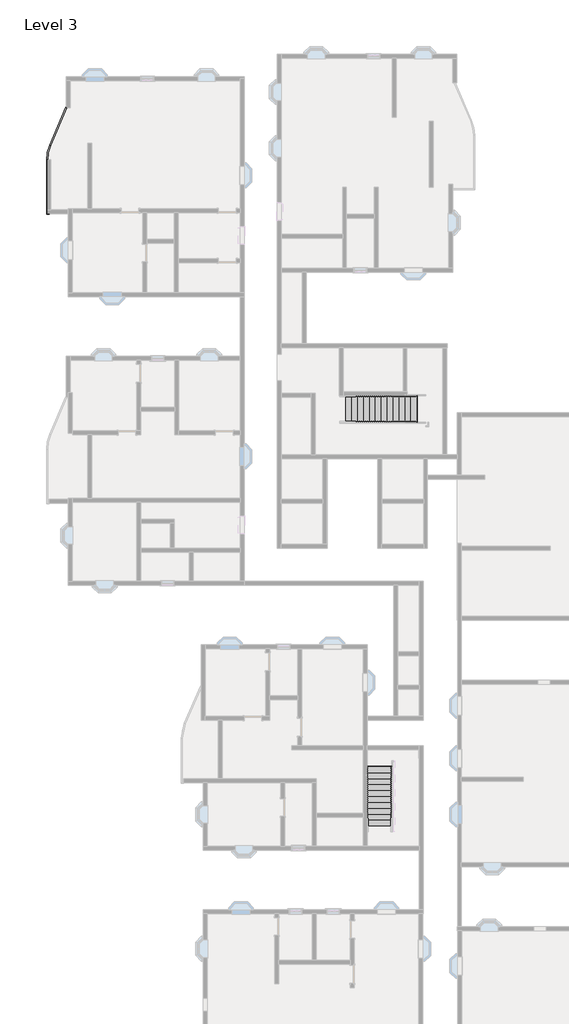
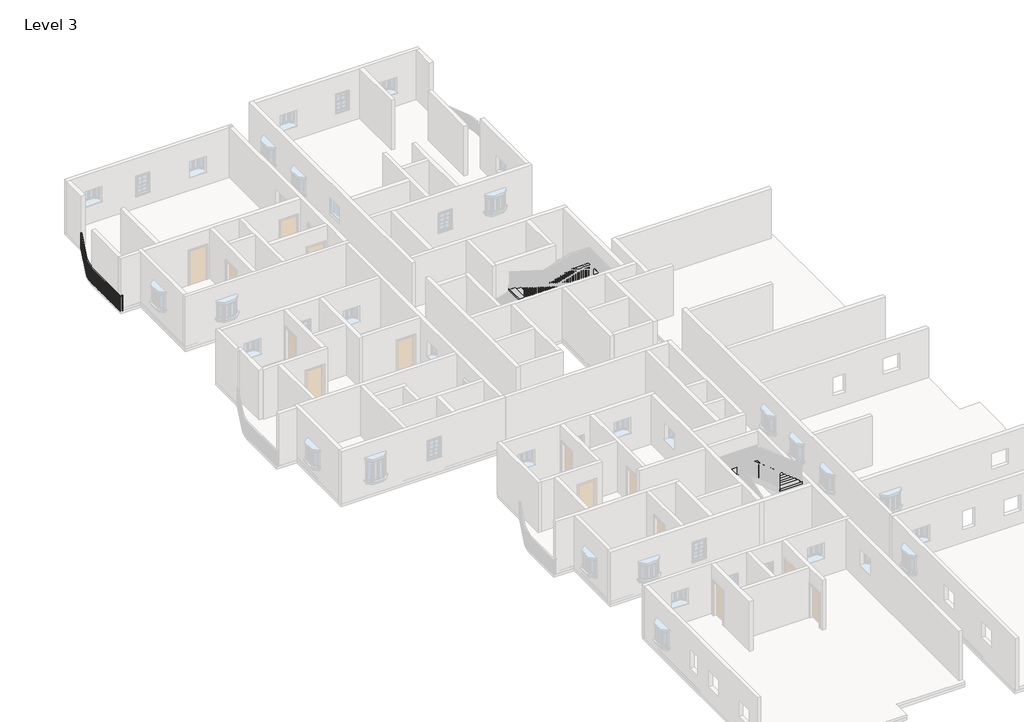
# One storey, part 12 of 14: 2 stair flights, 1 railing.
"""IFC4 building model written with IfcOpenShell, lengths in millimetres."""

from ifc_helpers import new_model, si_unit, frame, origin, place, context, project, spatial, polyline, circle_curve, outline, extrude, transform, mapped, element, save
from ifc_brep_helpers import plane_surface, cylinder_surface, revolved_surface, advanced_brep
from components import stair_flight_b14bcda7, stair_flight_b8102c9e

model = new_model("IFC4")

# Units and contexts
model_context = context("Model", 3, world=origin())
ifc_project = project(units=[si_unit("LENGTHUNIT", "METRE", prefix="MILLI")], contexts=[model_context])

# Site, building, storey
site = spatial("IfcSite", under=ifc_project)
building = spatial("IfcBuilding", under=site)
storey = spatial("IfcBuildingStorey", under=building, Name="Level 3", Elevation=6096.0)

# Railing
placement = place(None, origin())
element("IfcRailing", 1, ObjectType="Handrail - Rectangular", at=placement, inside=storey, context=model_context, shape_type="SolidModel", body=[
    advanced_brep(
    [(-19327.739878, 27355.8257339, 7010.4), (-19327.739878, 27355.8257339, 6959.6), (-19374.4383922, 27375.822953, 6959.6), (-19374.4383922, 27375.822953, 7010.4), (-20162.483418, 25406.4905323, 7010.4), (-20162.483418, 25406.4905323, 6959.6), (-20209.1819322, 25426.4877514, 6959.6), (-20209.1819322, 25426.4877514, 7010.4), (-20316.2891351, 24656.5948172, 6959.6), (-20316.2891351, 24656.5948172, 7010.4), (-20367.0891351, 24656.5948172, 6959.6), (-20367.0891351, 24656.5948172, 7010.4), (-20316.2891351, 21915.0583494, 7010.4), (-20316.2891351, 21915.0583494, 6959.6), (-20367.0891351, 21864.2583494, 6959.6), (-20367.0891351, 21864.2583494, 7010.4), (-20240.0891351, 21915.0583494, 7010.4), (-20240.0891351, 21864.2583494, 7010.4), (-20240.0891351, 21864.2583494, 6959.6), (-20240.0891351, 21915.0583494, 6959.6)],
    [
        (0, 1),
        (1, 2),
        (2, 3),
        (3, 0),
        (0, 4),
        (4, 5),
        (5, 1),
        (5, 6),
        (6, 2),
        (6, 7),
        (7, 3),
        (7, 4),
        (8, 5, circle_curve(frame((-18411.2891351, 24656.5948172, 6959.6), z_axis=(0.0, 0.0, -1.0), x_axis=(-0.9192620907623792, 0.3936460446736121, 0.0)), 1905.0)),
        (4, 9, circle_curve(frame((-18411.2891351, 24656.5948172, 7010.4), z_axis=(0.0, 0.0, 1.0), x_axis=(-0.9192620907623792, 0.3936460446736121, 0.0)), 1905.0)),
        (9, 8),
        (10, 6, circle_curve(frame((-18411.2891351, 24656.5948172, 6959.6), z_axis=(0.0, 0.0, -1.0), x_axis=(-0.9192620907623792, 0.3936460446736121, 0.0)), 1955.8)),
        (8, 10),
        (11, 7, circle_curve(frame((-18411.2891351, 24656.5948172, 7010.4), z_axis=(0.0, 0.0, -1.0), x_axis=(-0.9192620907623792, 0.3936460446736121, 0.0)), 1955.8)),
        (10, 11),
        (11, 9),
        (9, 12),
        (12, 13),
        (13, 8),
        (13, 14),
        (14, 10),
        (14, 15),
        (15, 11),
        (15, 12),
        (16, 17),
        (17, 18),
        (18, 19),
        (19, 16),
        (12, 16),
        (19, 13),
        (18, 14),
        (17, 15),
    ],
    [
        plane_surface(frame((-19351.0891351, 27365.8243434, 7010.4), z_axis=(0.3936460446736102, 0.91926209076238, 0.0), x_axis=(0.91926209076238, -0.3936460446736102, 0.0))),
        plane_surface(frame((-19327.739878, 27355.8257339, 7010.4), z_axis=(0.91926209076238, -0.3936460446736102, 0.0), x_axis=(-0.3936460446736102, -0.91926209076238, 0.0))),
        plane_surface(frame((-19327.739878, 27355.8257339, 6959.6), z_axis=(0.0, 0.0, -1.0), x_axis=(-0.3936460446736102, -0.91926209076238, 0.0))),
        plane_surface(frame((-19374.4383922, 27375.822953, 6959.6), z_axis=(-0.91926209076238, 0.3936460446736102, 0.0), x_axis=(-0.3936460446736102, -0.91926209076238, 0.0))),
        plane_surface(frame((-19374.4383922, 27375.822953, 7010.4), z_axis=(0.0, 0.0, 1.0), x_axis=(-0.3936460446736102, -0.91926209076238, 0.0))),
        revolved_surface(polyline([(-20162.48341800233, 25406.49053230323, 7010.4), (-20162.48341800233, 25406.49053230323, 6959.6)]), (-18411.2891351, 24656.5948172, 7010.4), (0.0, 0.0, 1.0)),
        plane_surface(frame((-18411.2891351, 24656.5948172, 6959.6), z_axis=(0.0, 0.0, -1.0), x_axis=(-0.9192620907623792, 0.3936460446736121, 0.0))),
        cylinder_surface(frame((-18411.2891351, 24656.5948172, 7010.4), z_axis=(0.0, 0.0, 1.0), x_axis=(-0.9192620907623792, 0.3936460446736121, 0.0)), 1955.8),
        plane_surface(frame((-18411.2891351, 24656.5948172, 7010.4), z_axis=(0.0, 0.0, 1.0), x_axis=(-0.9192620907623792, 0.3936460446736121, 0.0))),
        plane_surface(frame((-20316.2891351, 24656.5948172, 7010.4), z_axis=(1.0, 0.0, 0.0), x_axis=(0.0, -1.0, 0.0))),
        plane_surface(frame((-20316.2891351, 24656.5948172, 6959.6), z_axis=(0.0, 0.0, -1.0), x_axis=(0.0, -1.0, 0.0))),
        plane_surface(frame((-20367.0891351, 24656.5948172, 6959.6), z_axis=(-1.0, 0.0, 0.0), x_axis=(0.0, -1.0, 0.0))),
        plane_surface(frame((-20367.0891351, 24656.5948172, 7010.4), z_axis=(0.0, 0.0, 1.0), x_axis=(0.0, -1.0, 0.0))),
        plane_surface(frame((-20240.0891351, 21889.6583494, 7010.4), z_axis=(1.0, 0.0, 0.0), x_axis=(0.0, 1.0, 0.0))),
        plane_surface(frame((-20316.2891351, 21915.0583494, 7010.4), z_axis=(0.0, 1.0, 0.0), x_axis=(1.0, 0.0, 0.0))),
        plane_surface(frame((-20316.2891351, 21915.0583494, 6959.6), z_axis=(0.0, 0.0, -1.0), x_axis=(1.0, 0.0, 0.0))),
        plane_surface(frame((-20367.0891351, 21864.2583494, 6959.6), z_axis=(0.0, -1.0, 0.0), x_axis=(1.0, 0.0, 0.0))),
        plane_surface(frame((-20367.0891351, 21864.2583494, 7010.4), z_axis=(0.0, 0.0, 1.0), x_axis=(1.0, 0.0, 0.0))),
    ],
    [
        (0, [[1, 2, 3, 4]]),
        (1, [[-1, 5, 6, 7]]),
        (2, [[-2, -7, 8, 9]]),
        (3, [[-3, -9, 10, 11]]),
        (4, [[-4, -11, 12, -5]]),
        (5, [[13, -6, 14, 15]]),
        (6, [[16, -8, -13, 17]]),
        (7, [[18, -10, -16, 19]]),
        (8, [[-14, -12, -18, 20]]),
        (9, [[-15, 21, 22, 23]]),
        (10, [[-17, -23, 24, 25]]),
        (11, [[-19, -25, 26, 27]]),
        (12, [[-20, -27, 28, -21]]),
        (13, [[29, 30, 31, 32]]),
        (14, [[-22, 33, -32, 34]]),
        (15, [[-24, -34, -31, 35]]),
        (16, [[-26, -35, -30, 36]]),
        (17, [[-28, -36, -29, -33]]),
    ],
),
    extrude(outline(polyline([(-20351.2141351, 21922.9198172), (-20332.1641351, 21922.9198172), (-20332.1641351, 21903.8698172), (-20351.2141351, 21903.8698172), (-20351.2141351, 21922.9198172)])), frame((0.0, 0.0, 6096.0), z_axis=(0.0, 0.0, 1.0), x_axis=(1.0, 0.0, 0.0)), (0.0, 0.0, 1.0), 863.6),
    extrude(outline(polyline([(-20351.2141351, 22024.5198172), (-20332.1641351, 22024.5198172), (-20332.1641351, 22005.4698172), (-20351.2141351, 22005.4698172), (-20351.2141351, 22024.5198172)])), frame((0.0, 0.0, 6096.0), z_axis=(0.0, 0.0, 1.0), x_axis=(1.0, 0.0, 0.0)), (0.0, 0.0, 1.0), 863.6),
    extrude(outline(polyline([(-20351.2141351, 22126.1198172), (-20332.1641351, 22126.1198172), (-20332.1641351, 22107.0698172), (-20351.2141351, 22107.0698172), (-20351.2141351, 22126.1198172)])), frame((0.0, 0.0, 6096.0), z_axis=(0.0, 0.0, 1.0), x_axis=(1.0, 0.0, 0.0)), (0.0, 0.0, 1.0), 863.6),
    extrude(outline(polyline([(-20351.2141351, 22227.7198172), (-20332.1641351, 22227.7198172), (-20332.1641351, 22208.6698172), (-20351.2141351, 22208.6698172), (-20351.2141351, 22227.7198172)])), frame((0.0, 0.0, 6096.0), z_axis=(0.0, 0.0, 1.0), x_axis=(1.0, 0.0, 0.0)), (0.0, 0.0, 1.0), 863.6),
    extrude(outline(polyline([(-20351.2141351, 22329.3198172), (-20332.1641351, 22329.3198172), (-20332.1641351, 22310.2698172), (-20351.2141351, 22310.2698172), (-20351.2141351, 22329.3198172)])), frame((0.0, 0.0, 6096.0), z_axis=(0.0, 0.0, 1.0), x_axis=(1.0, 0.0, 0.0)), (0.0, 0.0, 1.0), 863.6),
    extrude(outline(polyline([(-20351.2141351, 22430.9198172), (-20332.1641351, 22430.9198172), (-20332.1641351, 22411.8698172), (-20351.2141351, 22411.8698172), (-20351.2141351, 22430.9198172)])), frame((0.0, 0.0, 6096.0), z_axis=(0.0, 0.0, 1.0), x_axis=(1.0, 0.0, 0.0)), (0.0, 0.0, 1.0), 863.6),
    extrude(outline(polyline([(-20351.2141351, 22532.5198172), (-20332.1641351, 22532.5198172), (-20332.1641351, 22513.4698172), (-20351.2141351, 22513.4698172), (-20351.2141351, 22532.5198172)])), frame((0.0, 0.0, 6096.0), z_axis=(0.0, 0.0, 1.0), x_axis=(1.0, 0.0, 0.0)), (0.0, 0.0, 1.0), 863.6),
    extrude(outline(polyline([(-20351.2141351, 22634.1198172), (-20332.1641351, 22634.1198172), (-20332.1641351, 22615.0698172), (-20351.2141351, 22615.0698172), (-20351.2141351, 22634.1198172)])), frame((0.0, 0.0, 6096.0), z_axis=(0.0, 0.0, 1.0), x_axis=(1.0, 0.0, 0.0)), (0.0, 0.0, 1.0), 863.6),
    extrude(outline(polyline([(-20351.2141351, 22735.7198172), (-20332.1641351, 22735.7198172), (-20332.1641351, 22716.6698172), (-20351.2141351, 22716.6698172), (-20351.2141351, 22735.7198172)])), frame((0.0, 0.0, 6096.0), z_axis=(0.0, 0.0, 1.0), x_axis=(1.0, 0.0, 0.0)), (0.0, 0.0, 1.0), 863.6),
    extrude(outline(polyline([(-20351.2141351, 22837.3198172), (-20332.1641351, 22837.3198172), (-20332.1641351, 22818.2698172), (-20351.2141351, 22818.2698172), (-20351.2141351, 22837.3198172)])), frame((0.0, 0.0, 6096.0), z_axis=(0.0, 0.0, 1.0), x_axis=(1.0, 0.0, 0.0)), (0.0, 0.0, 1.0), 863.6),
    extrude(outline(polyline([(-20351.2141351, 22938.9198172), (-20332.1641351, 22938.9198172), (-20332.1641351, 22919.8698172), (-20351.2141351, 22919.8698172), (-20351.2141351, 22938.9198172)])), frame((0.0, 0.0, 6096.0), z_axis=(0.0, 0.0, 1.0), x_axis=(1.0, 0.0, 0.0)), (0.0, 0.0, 1.0), 863.6),
    extrude(outline(polyline([(-20351.2141351, 23040.5198172), (-20332.1641351, 23040.5198172), (-20332.1641351, 23021.4698172), (-20351.2141351, 23021.4698172), (-20351.2141351, 23040.5198172)])), frame((0.0, 0.0, 6096.0), z_axis=(0.0, 0.0, 1.0), x_axis=(1.0, 0.0, 0.0)), (0.0, 0.0, 1.0), 863.6),
    extrude(outline(polyline([(-20351.2141351, 23142.1198172), (-20332.1641351, 23142.1198172), (-20332.1641351, 23123.0698172), (-20351.2141351, 23123.0698172), (-20351.2141351, 23142.1198172)])), frame((0.0, 0.0, 6096.0), z_axis=(0.0, 0.0, 1.0), x_axis=(1.0, 0.0, 0.0)), (0.0, 0.0, 1.0), 863.6),
    extrude(outline(polyline([(-20351.2141351, 23243.7198172), (-20332.1641351, 23243.7198172), (-20332.1641351, 23224.6698172), (-20351.2141351, 23224.6698172), (-20351.2141351, 23243.7198172)])), frame((0.0, 0.0, 6096.0), z_axis=(0.0, 0.0, 1.0), x_axis=(1.0, 0.0, 0.0)), (0.0, 0.0, 1.0), 863.6),
    extrude(outline(polyline([(-20351.2141351, 23345.3198172), (-20332.1641351, 23345.3198172), (-20332.1641351, 23326.2698172), (-20351.2141351, 23326.2698172), (-20351.2141351, 23345.3198172)])), frame((0.0, 0.0, 6096.0), z_axis=(0.0, 0.0, 1.0), x_axis=(1.0, 0.0, 0.0)), (0.0, 0.0, 1.0), 863.6),
    extrude(outline(polyline([(-20351.2141351, 23446.9198172), (-20332.1641351, 23446.9198172), (-20332.1641351, 23427.8698172), (-20351.2141351, 23427.8698172), (-20351.2141351, 23446.9198172)])), frame((0.0, 0.0, 6096.0), z_axis=(0.0, 0.0, 1.0), x_axis=(1.0, 0.0, 0.0)), (0.0, 0.0, 1.0), 863.6),
    extrude(outline(polyline([(-20351.2141351, 23548.5198172), (-20332.1641351, 23548.5198172), (-20332.1641351, 23529.4698172), (-20351.2141351, 23529.4698172), (-20351.2141351, 23548.5198172)])), frame((0.0, 0.0, 6096.0), z_axis=(0.0, 0.0, 1.0), x_axis=(1.0, 0.0, 0.0)), (0.0, 0.0, 1.0), 863.6),
    extrude(outline(polyline([(-20351.2141351, 23650.1198172), (-20332.1641351, 23650.1198172), (-20332.1641351, 23631.0698172), (-20351.2141351, 23631.0698172), (-20351.2141351, 23650.1198172)])), frame((0.0, 0.0, 6096.0), z_axis=(0.0, 0.0, 1.0), x_axis=(1.0, 0.0, 0.0)), (0.0, 0.0, 1.0), 863.6),
    extrude(outline(polyline([(-20351.2141351, 23751.7198172), (-20332.1641351, 23751.7198172), (-20332.1641351, 23732.6698172), (-20351.2141351, 23732.6698172), (-20351.2141351, 23751.7198172)])), frame((0.0, 0.0, 6096.0), z_axis=(0.0, 0.0, 1.0), x_axis=(1.0, 0.0, 0.0)), (0.0, 0.0, 1.0), 863.6),
    extrude(outline(polyline([(-20351.2141351, 23853.3198172), (-20332.1641351, 23853.3198172), (-20332.1641351, 23834.2698172), (-20351.2141351, 23834.2698172), (-20351.2141351, 23853.3198172)])), frame((0.0, 0.0, 6096.0), z_axis=(0.0, 0.0, 1.0), x_axis=(1.0, 0.0, 0.0)), (0.0, 0.0, 1.0), 863.6),
    extrude(outline(polyline([(-20351.2141351, 23954.9198172), (-20332.1641351, 23954.9198172), (-20332.1641351, 23935.8698172), (-20351.2141351, 23935.8698172), (-20351.2141351, 23954.9198172)])), frame((0.0, 0.0, 6096.0), z_axis=(0.0, 0.0, 1.0), x_axis=(1.0, 0.0, 0.0)), (0.0, 0.0, 1.0), 863.6),
    extrude(outline(polyline([(-20351.2141351, 24056.5198172), (-20332.1641351, 24056.5198172), (-20332.1641351, 24037.4698172), (-20351.2141351, 24037.4698172), (-20351.2141351, 24056.5198172)])), frame((0.0, 0.0, 6096.0), z_axis=(0.0, 0.0, 1.0), x_axis=(1.0, 0.0, 0.0)), (0.0, 0.0, 1.0), 863.6),
    extrude(outline(polyline([(-20351.2141351, 24158.1198172), (-20332.1641351, 24158.1198172), (-20332.1641351, 24139.0698172), (-20351.2141351, 24139.0698172), (-20351.2141351, 24158.1198172)])), frame((0.0, 0.0, 6096.0), z_axis=(0.0, 0.0, 1.0), x_axis=(1.0, 0.0, 0.0)), (0.0, 0.0, 1.0), 863.6),
    extrude(outline(polyline([(-20351.2141351, 24259.7198172), (-20332.1641351, 24259.7198172), (-20332.1641351, 24240.6698172), (-20351.2141351, 24240.6698172), (-20351.2141351, 24259.7198172)])), frame((0.0, 0.0, 6096.0), z_axis=(0.0, 0.0, 1.0), x_axis=(1.0, 0.0, 0.0)), (0.0, 0.0, 1.0), 863.6),
    extrude(outline(polyline([(-20351.2141351, 24361.3198172), (-20332.1641351, 24361.3198172), (-20332.1641351, 24342.2698172), (-20351.2141351, 24342.2698172), (-20351.2141351, 24361.3198172)])), frame((0.0, 0.0, 6096.0), z_axis=(0.0, 0.0, 1.0), x_axis=(1.0, 0.0, 0.0)), (0.0, 0.0, 1.0), 863.6),
    extrude(outline(polyline([(-20351.2141351, 24462.9198172), (-20332.1641351, 24462.9198172), (-20332.1641351, 24443.8698172), (-20351.2141351, 24443.8698172), (-20351.2141351, 24462.9198172)])), frame((0.0, 0.0, 6096.0), z_axis=(0.0, 0.0, 1.0), x_axis=(1.0, 0.0, 0.0)), (0.0, 0.0, 1.0), 863.6),
    extrude(outline(polyline([(-20351.2141351, 24564.5198172), (-20332.1641351, 24564.5198172), (-20332.1641351, 24545.4698172), (-20351.2141351, 24545.4698172), (-20351.2141351, 24564.5198172)])), frame((0.0, 0.0, 6096.0), z_axis=(0.0, 0.0, 1.0), x_axis=(1.0, 0.0, 0.0)), (0.0, 0.0, 1.0), 863.6),
    extrude(outline(polyline([(-20349.6005818, 24736.2720848), (-20330.5630441, 24735.5831307), (-20331.2519982, 24716.545593), (-20350.289536, 24717.2345471), (-20349.6005818, 24736.2720848)])), frame((0.0, 0.0, 6096.0), z_axis=(0.0, 0.0, 1.0), x_axis=(1.0, 0.0, 0.0)), (0.0, 0.0, 1.0), 863.6),
    extrude(outline(polyline([(-20342.724955, 24838.1310534), (-20323.750023, 24836.4415402), (-20325.4395363, 24817.4666081), (-20344.4144683, 24819.1561214), (-20342.724955, 24838.1310534)])), frame((0.0, 0.0, 6096.0), z_axis=(0.0, 0.0, 1.0), x_axis=(1.0, 0.0, 0.0)), (0.0, 0.0, 1.0), 863.6),
    extrude(outline(polyline([(-20330.5003254, 24939.4872677), (-20311.6405491, 24936.8018743), (-20314.3259425, 24917.942098), (-20333.1857188, 24920.6274914), (-20330.5003254, 24939.4872677)])), frame((0.0, 0.0, 6096.0), z_axis=(0.0, 0.0, 1.0), x_axis=(1.0, 0.0, 0.0)), (0.0, 0.0, 1.0), 863.6),
    extrude(outline(polyline([(-20312.9605484, 25040.0600272), (-20294.2681589, 25036.3861907), (-20297.9419954, 25017.6938012), (-20316.6343849, 25021.3676377), (-20312.9605484, 25040.0600272)])), frame((0.0, 0.0, 6096.0), z_axis=(0.0, 0.0, 1.0), x_axis=(1.0, 0.0, 0.0)), (0.0, 0.0, 1.0), 863.6),
    extrude(outline(polyline([(-20290.1541995, 25139.5708014), (-20271.6809643, 25134.9186963), (-20276.3330693, 25116.4454611), (-20294.8063045, 25121.0975662), (-20290.1541995, 25139.5708014)])), frame((0.0, 0.0, 6096.0), z_axis=(0.0, 0.0, 1.0), x_axis=(1.0, 0.0, 0.0)), (0.0, 0.0, 1.0), 863.6),
    extrude(outline(polyline([(-20262.1444395, 25237.7440008), (-20243.9415192, 25232.1265109), (-20249.5590091, 25213.9235906), (-20267.7619294, 25219.5410805), (-20262.1444395, 25237.7440008)])), frame((0.0, 0.0, 6096.0), z_axis=(0.0, 0.0, 1.0), x_axis=(1.0, 0.0, 0.0)), (0.0, 0.0, 1.0), 863.6),
    extrude(outline(polyline([(-20229.0088399, 25334.3077402), (-20211.1266465, 25327.7404228), (-20217.693964, 25309.8582293), (-20235.5761574, 25316.4255468), (-20229.0088399, 25334.3077402)])), frame((0.0, 0.0, 6096.0), z_axis=(0.0, 0.0, 1.0), x_axis=(1.0, 0.0, 0.0)), (0.0, 0.0, 1.0), 863.6),
    extrude(outline(polyline([(-20155.9843907, 25510.389225), (-20138.4724479, 25502.8902678), (-20145.9714051, 25485.378325), (-20163.4833479, 25492.8772822), (-20155.9843907, 25510.389225)])), frame((0.0, 0.0, 6096.0), z_axis=(0.0, 0.0, 1.0), x_axis=(1.0, 0.0, 0.0)), (0.0, 0.0, 1.0), 863.6),
    extrude(outline(polyline([(-20115.9899526, 25603.7862534), (-20098.4780098, 25596.2872963), (-20105.9769669, 25578.7753534), (-20123.4889098, 25586.2743106), (-20115.9899526, 25603.7862534)])), frame((0.0, 0.0, 6096.0), z_axis=(0.0, 0.0, 1.0), x_axis=(1.0, 0.0, 0.0)), (0.0, 0.0, 1.0), 863.6),
    extrude(outline(polyline([(-20075.9955145, 25697.1832818), (-20058.4835716, 25689.6843247), (-20065.9825288, 25672.1723818), (-20083.4944716, 25679.671339), (-20075.9955145, 25697.1832818)])), frame((0.0, 0.0, 6096.0), z_axis=(0.0, 0.0, 1.0), x_axis=(1.0, 0.0, 0.0)), (0.0, 0.0, 1.0), 863.6),
    extrude(outline(polyline([(-20036.0010763, 25790.5803103), (-20018.4891335, 25783.0813531), (-20025.9880906, 25765.5694103), (-20043.5000335, 25773.0683674), (-20036.0010763, 25790.5803103)])), frame((0.0, 0.0, 6096.0), z_axis=(0.0, 0.0, 1.0), x_axis=(1.0, 0.0, 0.0)), (0.0, 0.0, 1.0), 863.6),
    extrude(outline(polyline([(-19996.0066382, 25883.9773387), (-19978.4946954, 25876.4783815), (-19985.9936525, 25858.9664387), (-20003.5055953, 25866.4653958), (-19996.0066382, 25883.9773387)])), frame((0.0, 0.0, 6096.0), z_axis=(0.0, 0.0, 1.0), x_axis=(1.0, 0.0, 0.0)), (0.0, 0.0, 1.0), 863.6),
    extrude(outline(polyline([(-19956.0122, 25977.3743671), (-19938.5002572, 25969.8754099), (-19945.9992144, 25952.3634671), (-19963.5111572, 25959.8624243), (-19956.0122, 25977.3743671)])), frame((0.0, 0.0, 6096.0), z_axis=(0.0, 0.0, 1.0), x_axis=(1.0, 0.0, 0.0)), (0.0, 0.0, 1.0), 863.6),
    extrude(outline(polyline([(-19916.0177619, 26070.7713955), (-19898.5058191, 26063.2724384), (-19906.0047762, 26045.7604955), (-19923.5167191, 26053.2594527), (-19916.0177619, 26070.7713955)])), frame((0.0, 0.0, 6096.0), z_axis=(0.0, 0.0, 1.0), x_axis=(1.0, 0.0, 0.0)), (0.0, 0.0, 1.0), 863.6),
    extrude(outline(polyline([(-19876.0233238, 26164.1684239), (-19858.5113809, 26156.6694668), (-19866.0103381, 26139.157524), (-19883.5222809, 26146.6564811), (-19876.0233238, 26164.1684239)])), frame((0.0, 0.0, 6096.0), z_axis=(0.0, 0.0, 1.0), x_axis=(1.0, 0.0, 0.0)), (0.0, 0.0, 1.0), 863.6),
    extrude(outline(polyline([(-19836.0288856, 26257.5654524), (-19818.5169428, 26250.0664952), (-19826.0159, 26232.5545524), (-19843.5278428, 26240.0535095), (-19836.0288856, 26257.5654524)])), frame((0.0, 0.0, 6096.0), z_axis=(0.0, 0.0, 1.0), x_axis=(1.0, 0.0, 0.0)), (0.0, 0.0, 1.0), 863.6),
    extrude(outline(polyline([(-19796.0344475, 26350.9624808), (-19778.5225047, 26343.4635236), (-19786.0214618, 26325.9515808), (-19803.5334046, 26333.450538), (-19796.0344475, 26350.9624808)])), frame((0.0, 0.0, 6096.0), z_axis=(0.0, 0.0, 1.0), x_axis=(1.0, 0.0, 0.0)), (0.0, 0.0, 1.0), 863.6),
    extrude(outline(polyline([(-19756.0400094, 26444.3595092), (-19738.5280665, 26436.860552), (-19746.0270237, 26419.3486092), (-19763.5389665, 26426.8475664), (-19756.0400094, 26444.3595092)])), frame((0.0, 0.0, 6096.0), z_axis=(0.0, 0.0, 1.0), x_axis=(1.0, 0.0, 0.0)), (0.0, 0.0, 1.0), 863.6),
    extrude(outline(polyline([(-19716.0455712, 26537.7565376), (-19698.5336284, 26530.2575805), (-19706.0325855, 26512.7456376), (-19723.5445284, 26520.2445948), (-19716.0455712, 26537.7565376)])), frame((0.0, 0.0, 6096.0), z_axis=(0.0, 0.0, 1.0), x_axis=(1.0, 0.0, 0.0)), (0.0, 0.0, 1.0), 863.6),
    extrude(outline(polyline([(-19676.0511331, 26631.153566), (-19658.5391902, 26623.6546089), (-19666.0381474, 26606.1426661), (-19683.5500902, 26613.6416232), (-19676.0511331, 26631.153566)])), frame((0.0, 0.0, 6096.0), z_axis=(0.0, 0.0, 1.0), x_axis=(1.0, 0.0, 0.0)), (0.0, 0.0, 1.0), 863.6),
    extrude(outline(polyline([(-19636.0566949, 26724.5505945), (-19618.5447521, 26717.0516373), (-19626.0437093, 26699.5396945), (-19643.5556521, 26707.0386516), (-19636.0566949, 26724.5505945)])), frame((0.0, 0.0, 6096.0), z_axis=(0.0, 0.0, 1.0), x_axis=(1.0, 0.0, 0.0)), (0.0, 0.0, 1.0), 863.6),
    extrude(outline(polyline([(-19596.0622568, 26817.9476229), (-19578.550314, 26810.4486657), (-19586.0492711, 26792.9367229), (-19603.561214, 26800.4356801), (-19596.0622568, 26817.9476229)])), frame((0.0, 0.0, 6096.0), z_axis=(0.0, 0.0, 1.0), x_axis=(1.0, 0.0, 0.0)), (0.0, 0.0, 1.0), 863.6),
    extrude(outline(polyline([(-19556.0678187, 26911.3446513), (-19538.5558758, 26903.8456942), (-19546.054833, 26886.3337513), (-19563.5667758, 26893.8327085), (-19556.0678187, 26911.3446513)])), frame((0.0, 0.0, 6096.0), z_axis=(0.0, 0.0, 1.0), x_axis=(1.0, 0.0, 0.0)), (0.0, 0.0, 1.0), 863.6),
    extrude(outline(polyline([(-19516.0733805, 27004.7416797), (-19498.5614377, 26997.2427226), (-19506.0603948, 26979.7307797), (-19523.5723377, 26987.2297369), (-19516.0733805, 27004.7416797)])), frame((0.0, 0.0, 6096.0), z_axis=(0.0, 0.0, 1.0), x_axis=(1.0, 0.0, 0.0)), (0.0, 0.0, 1.0), 863.6),
    extrude(outline(polyline([(-19476.0789424, 27098.1387082), (-19458.5669996, 27090.639751), (-19466.0659567, 27073.1278082), (-19483.5778995, 27080.6267653), (-19476.0789424, 27098.1387082)])), frame((0.0, 0.0, 6096.0), z_axis=(0.0, 0.0, 1.0), x_axis=(1.0, 0.0, 0.0)), (0.0, 0.0, 1.0), 863.6),
    extrude(outline(polyline([(-19436.0845042, 27191.5357366), (-19418.5725614, 27184.0367794), (-19426.0715186, 27166.5248366), (-19443.5834614, 27174.0237937), (-19436.0845042, 27191.5357366)])), frame((0.0, 0.0, 6096.0), z_axis=(0.0, 0.0, 1.0), x_axis=(1.0, 0.0, 0.0)), (0.0, 0.0, 1.0), 863.6),
    extrude(outline(polyline([(-19396.0900661, 27284.932765), (-19378.5781233, 27277.4338078), (-19386.0770804, 27259.921865), (-19403.5890233, 27267.4208222), (-19396.0900661, 27284.932765)])), frame((0.0, 0.0, 6096.0), z_axis=(0.0, 0.0, 1.0), x_axis=(1.0, 0.0, 0.0)), (0.0, 0.0, 1.0), 863.6),
    extrude(outline(polyline([(-20351.2141351, 21899.1833494), (-20332.1641351, 21899.1833494), (-20332.1641351, 21880.1333494), (-20351.2141351, 21880.1333494), (-20351.2141351, 21899.1833494)])), frame((0.0, 0.0, 6096.0), z_axis=(0.0, 0.0, 1.0), x_axis=(1.0, 0.0, 0.0)), (0.0, 0.0, 1.0), 863.6),
    extrude(outline(polyline([(-20351.2141351, 24666.1198172), (-20332.1641351, 24666.1198172), (-20332.1641351, 24647.0698172), (-20351.2141351, 24647.0698172), (-20351.2141351, 24666.1198172)])), frame((0.0, 0.0, 6096.0), z_axis=(0.0, 0.0, 1.0), x_axis=(1.0, 0.0, 0.0)), (0.0, 0.0, 1.0), 863.6),
    extrude(outline(polyline([(-20190.839168, 25428.9945919), (-20173.3272251, 25421.4956347), (-20180.8261823, 25403.9836919), (-20198.3381251, 25411.482649), (-20190.839168, 25428.9945919)])), frame((0.0, 0.0, 6096.0), z_axis=(0.0, 0.0, 1.0), x_axis=(1.0, 0.0, 0.0)), (0.0, 0.0, 1.0), 863.6),
    extrude(outline(polyline([(-20259.1391351, 21880.1333494), (-20259.1391351, 21899.1833494), (-20240.0891351, 21899.1833494), (-20240.0891351, 21880.1333494), (-20259.1391351, 21880.1333494)])), frame((0.0, 0.0, 6096.0), z_axis=(0.0, 0.0, 1.0), x_axis=(1.0, 0.0, 0.0)), (0.0, 0.0, 1.0), 863.6),
    extrude(outline(polyline([(-19359.8451065, 27369.573822), (-19342.3331637, 27362.0748648), (-19349.8321209, 27344.562922), (-19367.3440637, 27352.0618792), (-19359.8451065, 27369.573822)])), frame((0.0, 0.0, 6096.0), z_axis=(0.0, 0.0, 1.0), x_axis=(1.0, 0.0, 0.0)), (0.0, 0.0, 1.0), 863.6),
])

# Stair flights
stair_flight_shape = stair_flight_b14bcda7(model_context)
element("IfcStairFlight", 2, ObjectType="2\" Tread 1\" Nosing 1/4\" Riser", at=placement, inside=storey, context=model_context, shape_type="MappedRepresentation", body=[
    mapped(stair_flight_shape, transform((0.0, 0.0, 0.0), x_axis=(1.0, 0.0, 0.0), y_axis=(0.0, 1.0, 0.0), z_axis=(0.0, 0.0, 1.0))),
])
stair_flight_2_shape = stair_flight_b8102c9e(model_context)
element("IfcStairFlight", 3, ObjectType="2\" Tread 1\" Nosing 1/4\" Riser", at=placement, inside=storey, context=model_context, shape_type="MappedRepresentation", body=[
    mapped(stair_flight_2_shape, transform((0.0, 0.0, 0.0), x_axis=(1.0, 0.0, 0.0), y_axis=(0.0, 1.0, 0.0), z_axis=(0.0, 0.0, 1.0))),
])

save(model, "model.ifc")

# Revit data of these elements
# Type "Handrail - Rectangular"
#   Assembly Code = "C2010400"
#   built-in parameter 1008612 = 0.0416667 (stored number, unit not read)
#   built-in parameter 1008611 = 0.0416667 (stored number, unit not read)
#   built-in parameter 1008609 = 0.333333 (stored number, unit not read)
#   built-in parameter 1008604 = 0.166667 (stored number, unit not read)
#   built-in parameter 1008603 = 0.166667 (stored number, unit not read)
#   Railing Height = 3' - 0"
#   built-in parameter 1008630 = 2
#   built-in parameter 1008610 = 2
#   built-in parameter 1008618 = Baluster - Square : 3/4"
# Element 1 (IfcRailing, "Handrail - Rectangular")
#   Phase Created = New Construction
# Elements 2, 3 (IfcStairFlight, "2\" Tread 1\" Nosing 1/4\" Riser")
#   Phase Created = New Construction
